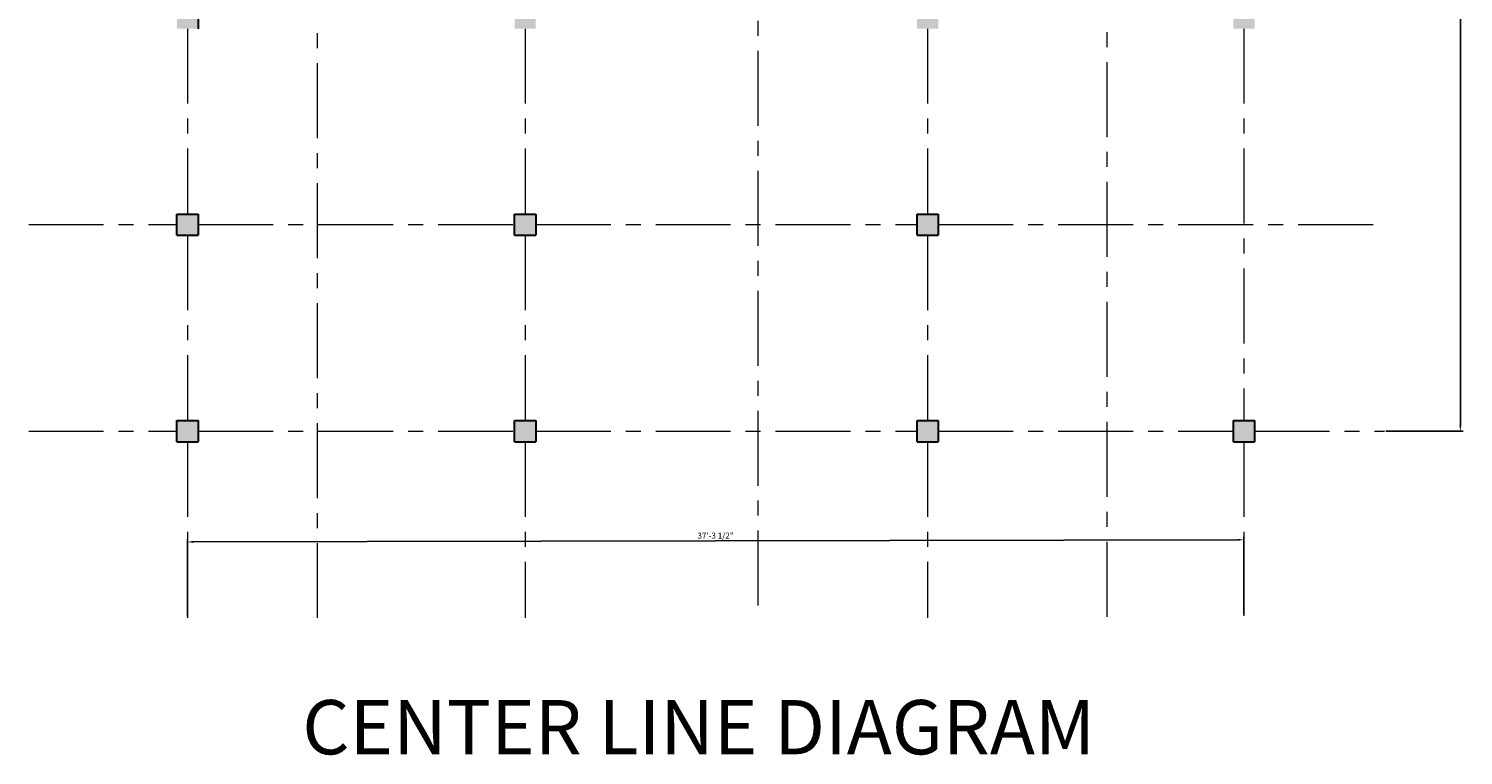
# Model space of a CAD drawing. Units: inches. Extents: x 4878 to 9282, y 5367 to 6617.
# Tile 7 of 14: x 5503 to 6111, y 5723 to 6031. Entities that reach past the tile are written whole.
import ezdxf

# ---------------------------------------------------------------- set-up
doc = ezdxf.new("R2010")
doc.units = ezdxf.units.IN
doc.linetypes.add('CENTER', pattern=[50.8, 31.75, -6.35, 6.35, -6.35])
for name, color, linetype, lineweight in [('A-ANNO-DIMS', 2, 'Continuous', 18), ('A-ANNO-TITL', 3, 'Continuous', 30), ('S-COLS', 1, 'Continuous', 30), ('S-COLS-PATT', 1, 'Continuous', 13), ('S-GRID', 4, 'CENTER', 13)]:
    doc.layers.add(name, color=color, linetype=linetype, lineweight=lineweight)
doc.styles.get("Standard").update_dxf_attribs({"font": 'arial.ttf'})
doc.dimstyles.new('ISO-25', dxfattribs={"dimtxt": 2.5, "dimasz": 2.5, "dimexe": 1.25, "dimexo": 0.625, "dimtad": 1, "dimdec": 0, "dimlunit": 3, "dimtxsty": 'Standard', "dimcen": 2.5, "dimadec": 0, "dimazin": 0, "dimtfac": 1, "dimtdec": 0, "dimtmove": 0, "dimatfit": 3, "dimfxl": 1, "dimarcsym": 0})

# ---------------------------------------------------------------- blocks, each defined once
blk = doc.blocks.new('COLUMN-9X9')
for p, q in [((0, 9), (9, 9)), ((0, 0), (0, 9)), ((9, 9), (9, 0)), ((0, 0), (9, 0))]:
    blk.add_line(p, q)
blk = doc.blocks.new('*D71')
at = {"layer": 'A-ANNO-DIMS', "color": 0, "lineweight": -2, "transparency": 16777216}
for p, q in [((5570.69, 5781.67), (5570.62, 5814.49)), ((5573.12, 5813.25), (6015.62, 5814.16)), ((6018.19, 5782.59), (6018.12, 5815.42))]:
    blk.add_line(p, q, dxfattribs=at)
at = {"layer": 'A-ANNO-DIMS', "color": 0, "transparency": 16777216}
for points in [[(5573.12, 5813.67), (5573.13, 5812.83), (5570.62, 5813.24)], [(6015.62, 5814.58), (6015.63, 5813.75), (6018.12, 5814.17)]]:
    blk.add_solid(points, dxfattribs=at)
at = {"layer": 'Defpoints', "color": 0, "transparency": 16777216}
for p in [(6018.12, 5814.17), (5570.69, 5781.04), (6018.19, 5781.97)]:
    blk.add_point(p, dxfattribs=at)
at = {"layer": 'A-ANNO-DIMS', "color": 0, "transparency": 16777216, "insert": (5794.37, 5815.62), "char_height": 2.5, "attachment_point": 5, "rotation": 0.11811}
blk.add_mtext('37\'-3 1/2"', dxfattribs=at)
blk = doc.blocks.new('*D78')
at = {"layer": 'A-ANNO-DIMS', "color": 0, "lineweight": -2, "transparency": 16777216}
for p, q in [((6078.26, 6314.14), (6111.09, 6314.14)), ((6109.84, 5862.64), (6109.84, 6311.64)), ((6078.26, 5860.14), (6111.09, 5860.14))]:
    blk.add_line(p, q, dxfattribs=at)
at = {"layer": 'A-ANNO-DIMS', "color": 0, "transparency": 16777216}
for points in [[(6109.42, 6311.64), (6110.26, 6311.64), (6109.84, 6314.14)], [(6109.42, 5862.64), (6110.26, 5862.64), (6109.84, 5860.14)]]:
    blk.add_solid(points, dxfattribs=at)
at = {"layer": 'Defpoints', "color": 0, "transparency": 16777216}
for p in [(6077.64, 6314.14), (6109.84, 6314.14), (6077.64, 5860.14)]:
    blk.add_point(p, dxfattribs=at)
at = {"layer": 'A-ANNO-DIMS', "color": 0, "transparency": 16777216, "insert": (6107.94, 6087.14), "char_height": 2.5, "attachment_point": 5, "rotation": 90}
blk.add_mtext('37\'-10"', dxfattribs=at)

msp = doc.modelspace()

# ---------------------------------------------------------------- hatches: boundary and pattern name
at = {"layer": 'S-COLS-PATT'}
h = msp.add_hatch(color=256, dxfattribs=at)
h.dxf.hatch_style = 1
h.paths.add_polyline_path([(5621.19, 6309.64), (5630.19, 6309.64), (5630.19, 6318.64), (5621.19, 6318.64)])
h.paths.add_polyline_path([(5718.19, 6318.64), (5709.19, 6318.64), (5709.19, 6309.64), (5718.19, 6309.64)])
h.paths.add_polyline_path([(5575.19, 6241.64), (5575.19, 6250.64), (5566.19, 6250.64), (5566.19, 6241.64)])
h.paths.add_polyline_path([(5709.19, 6241.92), (5718.19, 6241.92), (5718.19, 6250.92), (5709.19, 6250.92)])
h.paths.add_polyline_path([(5816.69, 6250.64), (5807.69, 6250.64), (5807.69, 6241.64), (5816.69, 6241.64)])
h.paths.add_polyline_path([(5888.69, 6250.64), (5879.69, 6250.64), (5879.69, 6241.64), (5888.69, 6241.64)])
h.paths.add_polyline_path([(5964.69, 6250.64), (5955.69, 6250.64), (5955.69, 6241.64), (5964.69, 6241.64)])
h.paths.add_polyline_path([(5718.19, 6182.64), (5709.19, 6182.64), (5709.19, 6173.64), (5718.19, 6173.64)])
h.paths.add_polyline_path([(5816.69, 6182.64), (5807.69, 6182.64), (5807.69, 6173.64), (5816.69, 6173.64)])
h.paths.add_polyline_path([(5888.69, 6182.64), (5879.69, 6182.64), (5879.69, 6173.64), (5888.69, 6173.64)])
h.paths.add_polyline_path([(6013.69, 6173.64), (6022.69, 6173.64), (6022.69, 6182.64), (6013.69, 6182.64)])
h.paths.add_polyline_path([(6022.69, 6039.64), (6013.69, 6039.64), (6013.69, 6030.64), (6022.69, 6030.64)])
h.paths.add_polyline_path([(5879.69, 6030.64), (5888.69, 6030.64), (5888.69, 6039.64), (5879.69, 6039.64)])
h.paths.add_polyline_path([(5718.19, 6103.64), (5709.19, 6103.64), (5709.19, 6094.64), (5718.19, 6094.64)])
h.paths.add_polyline_path([(5718.19, 6039.64), (5709.19, 6039.64), (5709.19, 6030.64), (5718.19, 6030.64)])
h.paths.add_polyline_path([(5575.19, 6039.64), (5566.19, 6039.64), (5566.19, 6030.64), (5575.19, 6030.64)])
h.paths.add_polyline_path([(5566.19, 6094.64), (5575.19, 6094.64), (5575.19, 6103.64), (5566.19, 6103.64)])
h.paths.add_polyline_path([(5566.19, 5943.14), (5575.19, 5943.14), (5575.19, 5952.14), (5566.19, 5952.14)])
h.paths.add_polyline_path([(5575.19, 5864.64), (5566.19, 5864.64), (5566.19, 5855.64), (5575.19, 5855.64)])
h.paths.add_polyline_path([(5709.19, 5943.14), (5718.19, 5943.14), (5718.19, 5952.14), (5709.19, 5952.14)])
h.paths.add_polyline_path([(5718.19, 5855.64), (5718.19, 5864.64), (5709.19, 5864.64), (5709.19, 5855.64)])
h.paths.add_polyline_path([(5879.69, 5855.64), (5888.69, 5855.64), (5888.69, 5864.64), (5879.69, 5864.64)])
h.paths.add_polyline_path([(6013.69, 5855.64), (6022.69, 5855.64), (6022.69, 5864.64), (6013.69, 5864.64)])
h.paths.add_polyline_path([(5888.69, 5952.14), (5879.69, 5952.14), (5879.69, 5943.14), (5888.69, 5943.14)])

# ---------------------------------------------------------------- linework, layer by layer
at = {"layer": 'S-COLS'}
msp.add_line((5575.19, 6039.64), (5575.19, 6030.64), dxfattribs=at)
at = {"layer": 'S-GRID'}
for p, q in [((5625.69, 5781.04), (5625.69, 6309.64)), ((5960.19, 5781.57), (5960.19, 6241.64)), ((5812.19, 6173.64), (5812.19, 5781.04)), ((5570.69, 6030.64), (5570.69, 5952.14)), ((5713.69, 6030.64), (5713.69, 5952.14)), ((5884.19, 6030.64), (5884.19, 5952.14)), ((6018.19, 6030.64), (6018.19, 5864.64)), ((5503.4, 5947.64), (5566.19, 5947.64)), ((5575.19, 5947.64), (5709.19, 5947.64)), ((5718.19, 5947.64), (5879.69, 5947.64)), ((5888.69, 5947.64), (6077.64, 5947.64)), ((5570.69, 5943.14), (5570.69, 5864.64)), ((5713.69, 5943.14), (5713.69, 5864.64)), ((5884.19, 5943.14), (5884.19, 5864.64)), ((5503.4, 5860.14), (5566.19, 5860.14)), ((5575.19, 5860.14), (5709.19, 5860.14)), ((5718.19, 5860.14), (5879.69, 5860.14)), ((5888.69, 5860.14), (6013.69, 5860.14)), ((6022.69, 5860.14), (6077.64, 5860.14)), ((5570.69, 5855.64), (5570.69, 5781.04)), ((5713.69, 5855.64), (5713.69, 5781.04)), ((5884.19, 5855.64), (5884.19, 5781.04)), ((6018.19, 5855.64), (6018.19, 5781.97))]:
    msp.add_line(p, q, dxfattribs=at)

# ---------------------------------------------------------------- block references
at = {"layer": 'S-COLS'}
for p in [(5566.19, 5943.15), (5709.19, 5943.15), (5879.69, 5943.15), (5566.19, 5855.64), (5709.19, 5855.64), (5879.69, 5855.64), (6013.69, 5855.64)]:
    msp.add_blockref('COLUMN-9X9', p, dxfattribs=at)

# ---------------------------------------------------------------- texts
at = {"layer": 'A-ANNO-TITL', "insert": (5619.29, 5746.29), "char_height": 23, "attachment_point": 1}
msp.add_mtext_dynamic_manual_height_columns('CENTER LINE DIAGRAM', width=1119.4399, gutter_width=12.5, heights=[0], dxfattribs=at)

# ---------------------------------------------------------------- dimensions: what is measured, and where the dimension line sits
at = {"layer": 'A-ANNO-DIMS'}
for base, p1, p2, angle, picture, middle in [((6109.84, 6314.14), (6077.64, 5860.14), (6077.64, 6314.14), 90, '*D78', (6107.94, 6087.14)), ((6018.12, 5814.17), (5570.69, 5781.04), (6018.19, 5781.97), 0.11811, '*D71', (5794.37, 5815.62))]:
    dim = msp.add_linear_dim(base=base, p1=p1, p2=p2, angle=angle, dimstyle='ISO-25', override={"dimdec": 1, "dimlfac": 1, "dimrnd": 0, "dimzin": 1, "dimdsep": 46, "dimlunit": 4, "dimfrac": 2}, dxfattribs=at)
    dim.commit()
    dim.dimension.update_dxf_attribs({"geometry": picture, "text_midpoint": middle})

doc.saveas('drawing.dxf')
